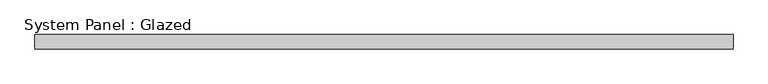
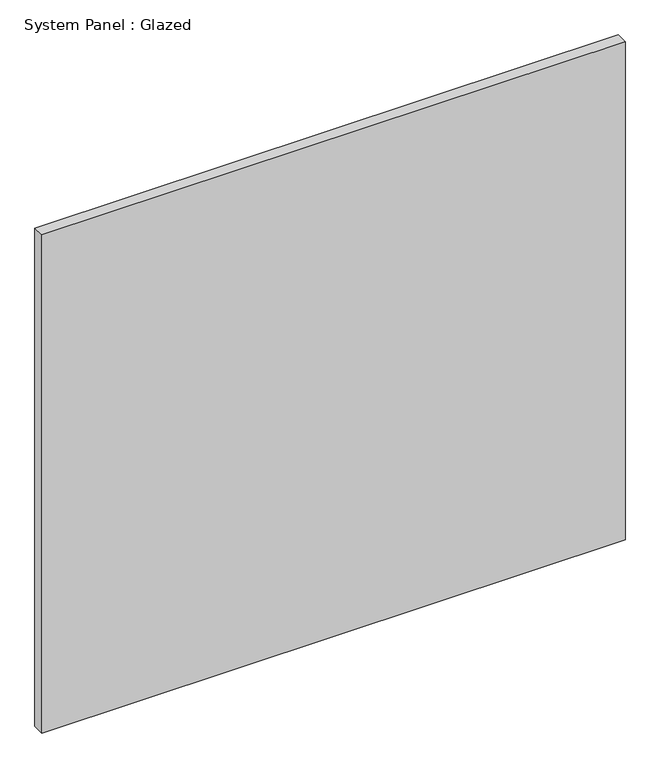
"""IFC4 building model written with IfcOpenShell, lengths in millimetres: plate geometry, System Panel : Glazed."""

from ifc_helpers import new_model, si_unit, origin, origin_with_axes, place, context, project, spatial, polyline, outline, extrude, source, transform, mapped, element, save


def system_panel_glazed_652821f2(model_context):
    return source(origin(), model_context, "Body", "SweptSolid", [
        extrude(outline(polyline([(622.3, 19.05), (-622.3, 19.05), (-622.3, 44.45), (622.3, 44.45), (622.3, 19.05)])), origin_with_axes(), (0.0, 0.0, 1.0), 1123.95),
    ])


if __name__ == "__main__":
    model = new_model("IFC4")
    model_context = context("Model", 3, world=origin())
    ifc_project = project(units=[si_unit("LENGTHUNIT", "METRE", prefix="MILLI")], contexts=[model_context])
    site = spatial("IfcSite", under=ifc_project)
    building = spatial("IfcBuilding", under=site)
    placement = place(None, origin())
    system_panel_glazed_shape = system_panel_glazed_652821f2(model_context)
    element("IfcPlate", 1, ObjectType="System Panel : Glazed", at=placement, inside=building, context=model_context, shape_type="MappedRepresentation", body=[
        mapped(system_panel_glazed_shape, transform((0.0, 0.0, 0.0), x_axis=(1.0, 0.0, 0.0), y_axis=(0.0, 1.0, 0.0), z_axis=(0.0, 0.0, 1.0))),
    ])
    save(model, "model.ifc")

# Revit data of these elements
# Type "System Panel : Glazed"
#   Construction Type Id = "GSP4R"
#   Analytic Construction = "1/8 in Pilkington single glazing"
#   Visual Light Transmittance = 0.9
#   Solar Heat Gain Coefficient = 0.86
#   Heat Transfer Coefficient (U) = 1.18115 BTU/(h·ft²·°F)
#   Define Thermal Properties by = 1
# Element 1 (IfcPlate, "System Panel : Glazed")
#   Materials on its faces: "Glass"
# Materials
#   "Glass": class "Glass", colour RGB 0 128 192, transparency 0.75, Description = "Soda Lime Glass", Cost = 0
